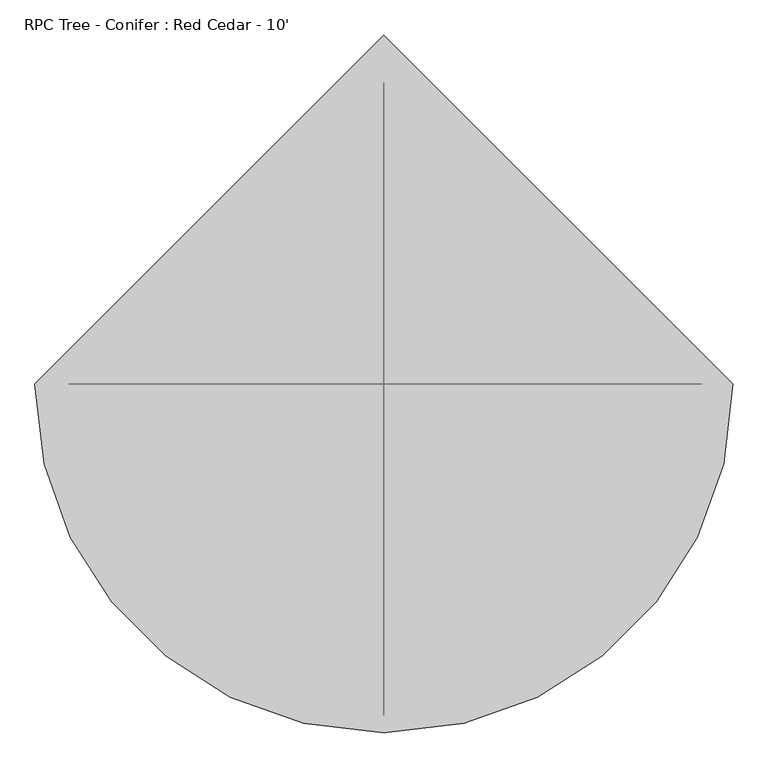
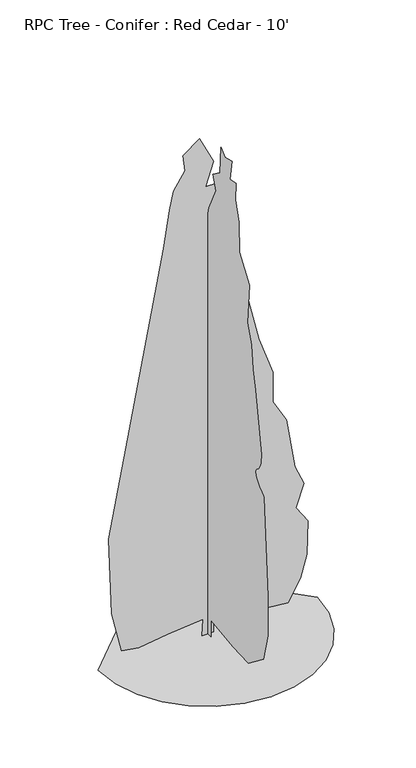
"""IFC4 building model written with IfcOpenShell, lengths in millimetres: geographic element geometry, RPC Tree - Conifer : Red Cedar - 10'."""

from ifc_helpers import new_model, si_unit, origin, place, context, project, spatial, triangles, source, transform, mapped, element, save


def rpc_tree_conifer_red_cedar_10_b4f4fd19(model_context):
    return source(origin(), model_context, "Body", "Tessellation", [
        triangles([(-33.3107415, 1.5e-06, 2.9e-06), (-28.1357486, -4.6e-06, 98.3225959), (-233.5175414, 5.5e-06, 79.3805562), (-399.6652124, 1.42e-05, 54.911224), (-499.0477364, 1.75e-05, 72.4481351), (-555.97166, 5.5e-06, 315.6659792), (-571.4961122, -2.13e-05, 776.2313261), (-483.5232479, -5.29e-05, 1241.968087), (-255.8301511, -0.0001341, 2437.3627087), (-219.6059632, -0.0001489, 2659.8870621), (-198.9065, -0.0001563, 2768.5481621), (-131.6330808, -0.0001654, 2872.0531815), (-141.9828215, -0.0001705, 2965.1948799), (-48.8352141, -0.0001789, 3037.6610962), (33.9626549, -0.0001727, 2872.0531815), (-12.6110955, -0.0001623, 2732.3276985), (49.4873863, -0.000165, 2732.3276985), (295.7992049, -0.0001139, 1694.3850941), (375.5044052, -0.0001037, 1464.4872082), (375.5044052, -9.29e-05, 1283.3674496), (453.1267748, -8.83e-05, 1148.821229), (504.8767047, -7.23e-05, 843.5031647), (556.6240911, -6.75e-05, 724.4813599), (510.0506621, -5.74e-05, 589.9350666), (577.3250805, -5.42e-05, 486.4377502), (572.1485796, -4.2e-05, 284.6170386), (535.9256453, -3.24e-05, 150.0712722), (463.4772695, -2.18e-05, 25.8744608), (342.1415071, -1.73e-05, 40.1411272), (173.6841841, -9.7e-06, 36.2241947), (33.9626549, -6.7e-06, 87.9728642), (33.9626549, -1.5e-06, 0.0), (0.1966724, 29.3359728, 9.21e-05), (0.1966704, 39.6857044, 72.4483894), (0.1966774, 118.2140961, 25.2313837), (0.1966799, 262.2040898, 67.2733964), (0.1966804, 231.1559123, 108.6723366), (0.1966888, 422.6253662, 108.6723366), (0.1966933, 505.4242367, 129.3717999), (0.1966992, 520.9487251, 248.3938681), (0.1967042, 546.8236719, 465.7393044), (0.1967063, 510.5982305, 548.5356314), (0.1967124, 515.7747313, 683.0819246), (0.1967146, 479.5492536, 771.0548252), (0.1967186, 464.0248014, 1003.9244047), (0.1967195, 396.7529265, 1091.8973053), (0.1967291, 303.6035432, 1531.7615902), (0.1967344, 200.1064449, 1883.6530472), (0.196737, 127.6585687, 2142.3977188), (0.1967365, 91.4343717, 2168.2701221), (0.1967411, 60.3851723, 2302.8164154), (0.1967457, -12.0630389, 2608.147197), (0.1967489, -84.5113568, 2753.0287605), (0.1967483, -53.4621528, 2835.8327179), (0.1967476, -120.7355538, 2887.572583), (0.1967542, -131.0852854, 3047.9988373), (0.1967508, -172.484221, 3011.7783737), (0.1967485, -239.7573677, 3027.2977753), (0.196744, -224.2328974, 2908.2733543), (0.1967419, -281.1575659, 2918.6366753), (0.1967377, -275.9810469, 2815.1316559), (0.1967366, -312.2065247, 2701.2888954), (0.1967285, -317.3804821, 2520.1615791), (0.1967235, -419.0363411, 2380.6522167), (0.1967139, -395.0028517, 2137.2211452), (0.1967074, -436.4023232, 2028.5498714), (0.1967061, -451.9267754, 1888.8270046), (0.1967, -477.8017585, 1774.9817734), (0.1966875, -534.7256822, 1417.9137428), (0.1966867, -534.5885176, 1400.1872086), (0.196686, -533.6385392, 1382.5493317), (0.1966853, -531.0579191, 1365.0945831), (0.1966848, -526.0338072, 1347.911475), (0.1966844, -517.7508462, 1331.0889553), (0.1966843, -505.3962951, 1314.7187336), (0.1966843, -488.1522532, 1298.891938), (0.196684, -477.659507, 1280.543058), (0.1966828, -482.7217343, 1258.2012531), (0.196681, -498.2538168, 1234.3506741), (0.1966791, -519.178339, 1211.4779423), (0.1966774, -540.4152695, 1192.0621943), (0.1966761, -556.8820696, 1178.5925222), (0.1966811, -563.4987805, 1173.5481354), (0.1966595, -601.9975571, 589.9350666), (0.1966546, -601.9975571, 351.891457), (0.1966492, -555.4241281, 181.1204671), (0.1966508, -405.3533463, 67.2733964), (0.1966578, -250.1068449, 72.4481351), (0.1966686, -32.7624306, 103.4973345), (0.1966697, -32.7624306, 8.84e-05), (-633.2080067, 0.0, 0.000118), (-616.4617905, -145.1342734, 0.0001086), (-568.7732406, -278.4169084, 9.86e-05), (-493.955024, -396.0290245, 8.83e-05), (-395.8323432, -494.1517053, 7.82e-05), (-278.2202452, -568.9699219, 6.86e-05), (-144.9376012, -616.6584354, 5.99e-05), (0.1966989, -633.4046516, 5.26e-05), (145.3309457, -616.6584354, 4.72e-05), (278.6135715, -568.9699219, 0.0001331), (396.2257058, -494.1517053, 0.0001324), (494.35093, -396.0290245, 0.0001339), (569.1666032, -278.4169084, 4.88e-05), (616.8550804, -145.1342734, 5.47e-05), (633.6012966, 5.54e-05, 6.26e-05), (0.1965877, 633.4046516, 0.0001281)], [[13, 14, 15], [12, 13, 15], [12, 15, 16], [11, 12, 16], [32, 1, 2], [31, 32, 2], [10, 11, 16], [16, 17, 18], [10, 16, 18], [9, 10, 18], [8, 9, 18], [8, 18, 19], [8, 19, 20], [7, 8, 20], [7, 20, 21], [7, 21, 22], [6, 7, 22], [6, 22, 23], [6, 23, 24], [5, 6, 24], [4, 5, 24], [3, 4, 24], [2, 3, 24], [31, 2, 24], [30, 31, 24], [29, 30, 24], [29, 24, 25], [29, 25, 26], [29, 26, 27], [29, 27, 28], [55, 56, 57], [35, 36, 37], [57, 58, 59], [55, 57, 59], [59, 60, 61], [89, 90, 33], [89, 33, 34], [53, 54, 55], [55, 59, 61], [53, 55, 61], [53, 61, 62], [52, 53, 62], [52, 62, 63], [51, 52, 63], [51, 63, 64], [51, 64, 65], [50, 51, 65], [38, 39, 40], [34, 35, 37], [50, 65, 66], [50, 66, 67], [49, 50, 67], [48, 49, 67], [48, 67, 68], [47, 48, 68], [47, 68, 69], [46, 47, 69], [46, 69, 70], [46, 70, 71], [46, 71, 72], [46, 72, 73], [46, 73, 74], [46, 74, 75], [46, 75, 76], [46, 76, 77], [46, 77, 78], [46, 78, 79], [46, 79, 80], [37, 38, 40], [37, 40, 41], [37, 41, 42], [46, 80, 81], [82, 83, 84], [34, 37, 42], [89, 34, 42], [89, 42, 43], [89, 43, 44], [45, 46, 81], [44, 45, 81], [89, 44, 81], [88, 89, 81], [88, 81, 82], [88, 82, 84], [88, 84, 85], [88, 85, 86], [88, 86, 87], [105, 106, 91], [104, 105, 91], [104, 91, 92], [103, 104, 92], [103, 92, 93], [103, 93, 94], [102, 103, 94], [101, 102, 94], [101, 94, 95], [101, 95, 96], [101, 96, 97], [101, 97, 98], [101, 98, 99], [101, 99, 100]], closed=False),
    ])


if __name__ == "__main__":
    model = new_model("IFC4")
    model_context = context("Model", 3, world=origin())
    ifc_project = project(units=[si_unit("LENGTHUNIT", "METRE", prefix="MILLI")], contexts=[model_context])
    site = spatial("IfcSite", under=ifc_project)
    building = spatial("IfcBuilding", under=site)
    placement = place(None, origin())
    rpc_tree_conifer_red_cedar_10_shape = rpc_tree_conifer_red_cedar_10_b4f4fd19(model_context)
    element("IfcGeographicElement", 1, ObjectType="RPC Tree - Conifer : Red Cedar - 10'", at=placement, inside=building, context=model_context, shape_type="MappedRepresentation", body=[
        mapped(rpc_tree_conifer_red_cedar_10_shape, transform((0.0, 0.0, 0.0), x_axis=(1.0, 0.0, 0.0), y_axis=(0.0, 1.0, 0.0), z_axis=(0.0, 0.0, 1.0))),
    ])
    save(model, "model.ifc")

# Revit data of these elements
# Type "RPC Tree - Conifer : Red Cedar - 10'"
#   built-in parameter 1005198 = "{2, 15},{39, RPC-16-FXGH-CPG0-PPQ3-C000-ST1L-LVER-AU},{1, 0},{1, 0},{2, 13},{1, 8},{5, Color},{1, 0},{1, 0},{3, 0.8},{3, 0.8},{3, 0.8},{1, 8},{7, BBoxMin},{1, 0},{1, 0},{1, 0},{1, 0},{1, 0},{1, 8},{7, BBoxMax},{1, 0},{1, 0},{1, 0},{1, 0},{1, 0},{2, 11},{9, RPCTypeId},{1, 0},{1, 0},{39, RPC-16-FXGH-CPG0-PPQ3-C000-ST1L-LVER-AU},{1, 6},{14, RPCPlantHeight},{1, 0},{1, 0},{2, 10},{2, 11},{7, keyword},{1, 0},{1, 0},{34, :RPCs:Trees [General]:Geometry:RPC},{2, 11},{8, category},{1, 0},{1, 0},{15, Trees [General]},{2, 11},{12, LocalizedUID},{1, 0},{1, 0},{9, Red Cedar},{2, 14},{6, Height},{1, 0},{1, 0},{2, 10},{1, 2},{16, Cast Reflections},{1, 0},{1, 0},{1, 0},{1, 2},{12, Cast Shadows},{1, 0},{1, 0},{1, 1},{1, 2},{9, Lock View},{1, 0},{1, 0},{1, 0},{1, 4},{5, ViewC},{1, 0},{1, 0},{1, 0},{21, assetlibrary_base.fbx},{1, 5},"
#   built-in parameter 1005195 = "RPC-16-FXGH-CPG0-PPQ3-C000-ST1L-LVER-AU"
#   Type Comments = "Red Cedar"
#   Assembly Code = "G2050500"
#   Height = 10' - 0"
#   Description = (empty or 0)
#   Default Elevation = 0
